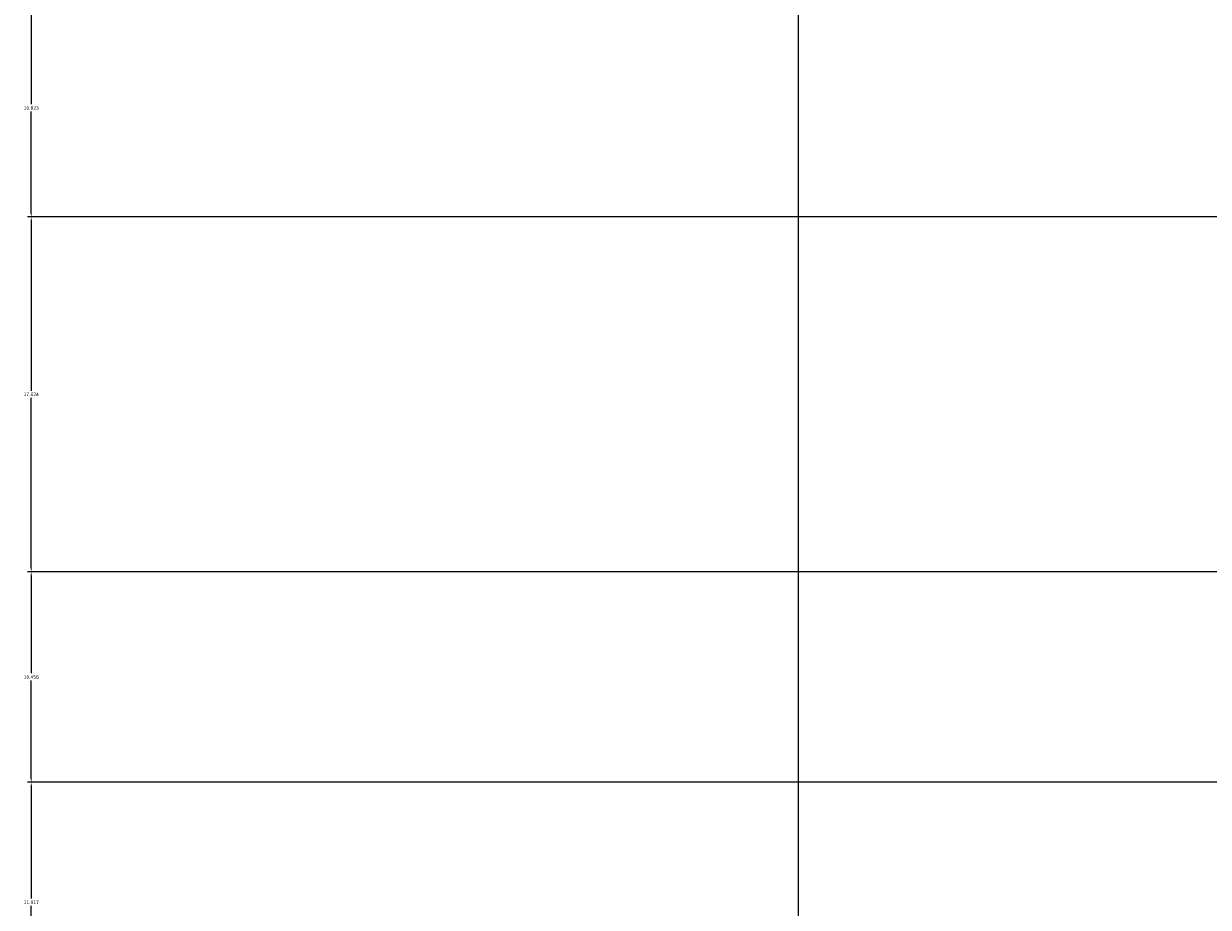
# Model space of a CAD drawing. Units: inches. Extents: x 412 to 584, y 208 to 437.
# Tile 15 of 28: x 412 to 471, y 315 to 359. Entities that reach past the tile are written whole.
import ezdxf

# ---------------------------------------------------------------- set-up
doc = ezdxf.new("R2010")
doc.units = ezdxf.units.IN
doc.header["$MEASUREMENT"] = 0
doc.layers.add('A-ANNO-DIMS', color=2, linetype='Continuous', lineweight=18)
doc.styles.get("Standard").update_dxf_attribs({"font": 'arial.ttf'})
doc.dimstyles.get("Standard").update_dxf_attribs({"dimtxt": 0.18, "dimasz": 0.18, "dimexe": 0.18, "dimexo": 0.0625, "dimgap": 0.09, "dimtad": 0, "dimtih": 1, "dimtoh": 1, "dimdec": 4, "dimzin": 0, "dimdsep": 46, "dimtxsty": 'Standard', "dimcen": 0.09, "dimadec": 0, "dimazin": 0, "dimtfac": 1, "dimtdec": 4, "dimtofl": 0, "dimtmove": 0, "dimatfit": 3, "dimfxl": 1, "dimtolj": 1, "dimtzin": 0, "dimarcsym": 0})

# ---------------------------------------------------------------- blocks, each defined once
blk = doc.blocks.new('*D23')
at = {"layer": 'A-ANNO-DIMS', "color": 0, "lineweight": -2, "transparency": 16777216}
for p, q in [((466.041, 360.196), (412.276, 360.196)), ((412.456, 360.016), (412.456, 354.967)), ((412.456, 349.553), (412.456, 354.603)), ((499.225, 349.373), (412.276, 349.373))]:
    blk.add_line(p, q, dxfattribs=at)
at = {"layer": 'A-ANNO-DIMS', "color": 0, "transparency": 16777216}
for points in [[(412.426, 360.016), (412.486, 360.016), (412.456, 360.196)], [(412.426, 349.553), (412.486, 349.553), (412.456, 349.373)]]:
    blk.add_solid(points, dxfattribs=at)
at = {"layer": 'Defpoints', "color": 0, "transparency": 16777216}
for p in [(466.104, 360.196), (412.456, 349.373), (499.288, 349.373)]:
    blk.add_point(p, dxfattribs=at)
at = {"layer": 'A-ANNO-DIMS', "color": 0, "transparency": 16777216, "insert": (412.456, 354.785), "char_height": 0.18, "attachment_point": 5}
blk.add_mtext('\\A1;10.823', dxfattribs=at)
blk = doc.blocks.new('*D24')
at = {"layer": 'A-ANNO-DIMS', "color": 0, "lineweight": -2, "transparency": 16777216}
for p, q in [((499.225, 349.373), (412.276, 349.373)), ((412.456, 349.193), (412.456, 340.743)), ((412.456, 331.93), (412.456, 340.38)), ((499.225, 331.75), (412.276, 331.75))]:
    blk.add_line(p, q, dxfattribs=at)
at = {"layer": 'A-ANNO-DIMS', "color": 0, "transparency": 16777216}
for points in [[(412.426, 349.193), (412.486, 349.193), (412.456, 349.373)], [(412.426, 331.93), (412.486, 331.93), (412.456, 331.75)]]:
    blk.add_solid(points, dxfattribs=at)
at = {"layer": 'Defpoints', "color": 0, "transparency": 16777216}
for p in [(499.288, 349.373), (412.456, 331.75), (499.288, 331.75)]:
    blk.add_point(p, dxfattribs=at)
at = {"layer": 'A-ANNO-DIMS', "color": 0, "transparency": 16777216, "insert": (412.456, 340.561), "char_height": 0.18, "attachment_point": 5}
blk.add_mtext('\\A1;17.624', dxfattribs=at)
blk = doc.blocks.new('*D25')
at = {"layer": 'A-ANNO-DIMS', "color": 0, "lineweight": -2, "transparency": 16777216}
for p, q in [((499.225, 331.75), (412.276, 331.75)), ((412.456, 331.57), (412.456, 326.704)), ((412.456, 321.474), (412.456, 326.34)), ((499.225, 321.294), (412.276, 321.294))]:
    blk.add_line(p, q, dxfattribs=at)
at = {"layer": 'A-ANNO-DIMS', "color": 0, "transparency": 16777216}
for points in [[(412.426, 331.57), (412.486, 331.57), (412.456, 331.75)], [(412.426, 321.474), (412.486, 321.474), (412.456, 321.294)]]:
    blk.add_solid(points, dxfattribs=at)
at = {"layer": 'Defpoints', "color": 0, "transparency": 16777216}
for p in [(499.288, 331.75), (412.456, 321.294), (499.288, 321.294)]:
    blk.add_point(p, dxfattribs=at)
at = {"layer": 'A-ANNO-DIMS', "color": 0, "transparency": 16777216, "insert": (412.456, 326.522), "char_height": 0.18, "attachment_point": 5}
blk.add_mtext('\\A1;10.456', dxfattribs=at)
blk = doc.blocks.new('*D26')
at = {"layer": 'A-ANNO-DIMS', "color": 0, "lineweight": -2, "transparency": 16777216}
for p, q in [((499.225, 321.294), (412.276, 321.294)), ((412.456, 321.114), (412.456, 315.518)), ((412.456, 309.557), (412.456, 315.154)), ((423.494, 309.377), (412.276, 309.377))]:
    blk.add_line(p, q, dxfattribs=at)
at = {"layer": 'A-ANNO-DIMS', "color": 0, "transparency": 16777216}
for points in [[(412.426, 321.114), (412.486, 321.114), (412.456, 321.294)], [(412.426, 309.557), (412.486, 309.557), (412.456, 309.377)]]:
    blk.add_solid(points, dxfattribs=at)
at = {"layer": 'Defpoints', "color": 0, "transparency": 16777216}
for p in [(499.288, 321.294), (412.456, 309.377), (423.556, 309.377)]:
    blk.add_point(p, dxfattribs=at)
at = {"layer": 'A-ANNO-DIMS', "color": 0, "transparency": 16777216, "insert": (412.456, 315.336), "char_height": 0.18, "attachment_point": 5}
blk.add_mtext('\\A1;11.917', dxfattribs=at)
blk = doc.blocks.new('*D28')
at = {"layer": 'A-ANNO-DIMS', "color": 0, "lineweight": -2, "transparency": 16777216}
for p, q in [((450.562, 256.635), (450.562, 437.465)), ((450.742, 437.285), (502.724, 437.285)), ((555.616, 437.285), (503.634, 437.285)), ((555.796, 256.635), (555.796, 437.465))]:
    blk.add_line(p, q, dxfattribs=at)
at = {"layer": 'A-ANNO-DIMS', "color": 0, "transparency": 16777216}
for points in [[(450.742, 437.315), (450.742, 437.255), (450.562, 437.285)], [(555.616, 437.315), (555.616, 437.255), (555.796, 437.285)]]:
    blk.add_solid(points, dxfattribs=at)
at = {"layer": 'Defpoints', "color": 0, "transparency": 16777216}
for p in [(555.796, 437.285), (450.562, 256.573), (555.796, 256.573)]:
    blk.add_point(p, dxfattribs=at)
at = {"layer": 'A-ANNO-DIMS', "color": 0, "transparency": 16777216, "insert": (503.179, 437.285), "char_height": 0.18, "attachment_point": 5}
blk.add_mtext('\\A1;105.23', dxfattribs=at)

msp = doc.modelspace()

# ---------------------------------------------------------------- dimensions: what is measured, and where the dimension line sits
at = {"layer": 'A-ANNO-DIMS'}
dim = msp.add_linear_dim(base=(555.7959, 437.2847), p1=(450.562, 256.5729), p2=(555.7959, 256.5729), dimstyle='Standard', override={"dimdec": 2, "dimlfac": 1, "dimrnd": 0, "dimzin": 0, "dimdsep": 46, "dimlunit": 2}, dxfattribs=at)
dim.commit()
dim.dimension.update_dxf_attribs({"geometry": '*D28', "text_midpoint": (503.1789, 437.2847)})
for base, p1, p2, picture, middle in [((412.4562, 349.3734), (466.1037, 360.1961), (499.2878, 349.3734), '*D23', (412.4562, 354.7847)), ((412.4562, 331.7496), (499.2878, 349.3734), (499.2878, 331.7496), '*D24', (412.4562, 340.5615)), ((412.45622, 321.29408), (499.28783, 331.74962), (499.28783, 321.29408), '*D25', (412.45622, 326.52185)), ((412.4562, 309.3773), (499.2878, 321.2941), (423.5562, 309.3773), '*D26', (412.4562, 315.3357))]:
    dim = msp.add_linear_dim(base=base, p1=p1, p2=p2, angle=90, dimstyle='Standard', override={"dimdec": 3, "dimlfac": 1, "dimrnd": 0, "dimzin": 0, "dimdsep": 46, "dimlunit": 2}, dxfattribs=at)
    dim.commit()
    dim.dimension.update_dxf_attribs({"geometry": picture, "text_midpoint": middle})

doc.saveas('drawing.dxf')
